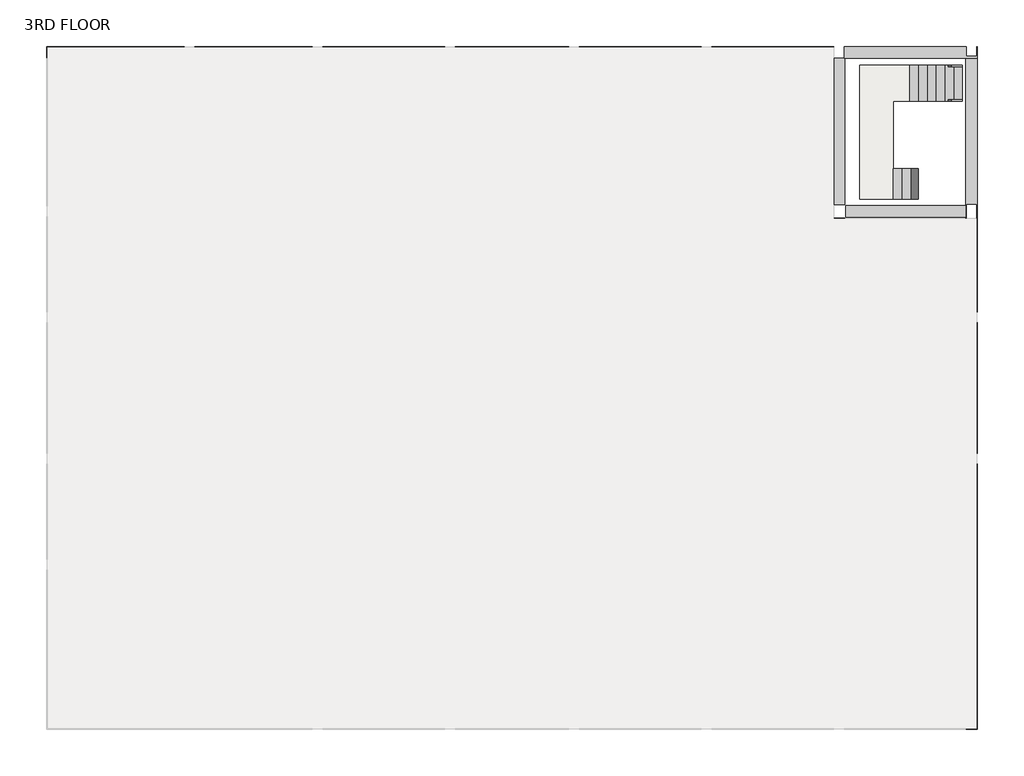
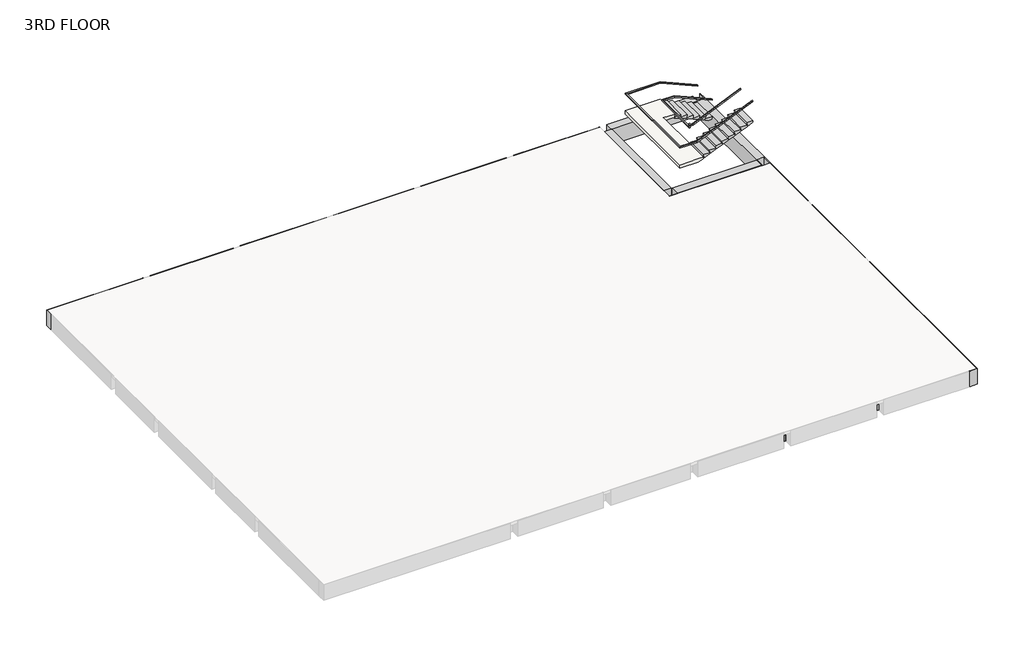
# One storey, part 2 of 2: 5 beams, 2 railings, 2 stair flights, 1 slab.
"""IFC4 building model written with IfcOpenShell, lengths in millimetres."""

from ifc_helpers import new_model, si_unit, frame, origin, place, context, project, spatial, polyline, outline, extrude, faceted_brep, element, save

model = new_model("IFC4")

# Units and contexts
model_context = context("Model", 3, world=origin())
ifc_project = project(units=[si_unit("LENGTHUNIT", "METRE", prefix="MILLI")], contexts=[model_context])

# Site, building, storey
site = spatial("IfcSite", under=ifc_project)
building = spatial("IfcBuilding", under=site)
storey = spatial("IfcBuildingStorey", under=building, Name="3RD FLOOR", Elevation=10668.0)

# Beams
placement = place(None, origin())
element("IfcBeam", 1, ObjectType="M_Concrete-Rectangular Beam : 400 x 800mm", at=placement, inside=storey, context=model_context, shape_type="Brep", body=[
    faceted_brep([(6397.6508981, 16716.9690835, 10668.0), (6397.6508981, 17116.9690835, 10668.0), (6375.4508981, 17116.9690835, 10668.0), (6375.4508981, 16789.9690835, 10668.0), (6019.8508981, 16789.9690835, 10668.0), (6019.8508981, 17116.9690835, 10668.0), (1803.4508981, 17116.9690835, 10668.0), (1803.4508981, 16716.9690835, 10668.0), (1825.6508981, 16716.9690835, 10668.0), (5997.6508981, 16716.9690835, 10668.0), (6397.6508981, 16716.9690835, 9868.0), (1803.4508981, 16716.9690835, 9868.0), (1825.6508981, 16716.9690835, 9868.0), (5997.6508981, 16716.9690835, 9868.0), (6397.6508981, 17116.9690835, 9868.0), (1803.4508981, 17116.9690835, 9868.0), (6019.8508981, 17116.9690835, 9868.0), (6019.8508981, 16789.9690835, 9868.0), (6375.4508981, 16789.9690835, 9868.0), (6375.4508981, 17116.9690835, 9868.0)], [[[0, 1, 2, 3, 4, 5, 6, 7, 8, 9]], [[10, 0, 9, 8, 7, 11, 12, 13]], [[14, 10, 13, 12, 11, 15, 16, 17, 18, 19]], [[1, 14, 19, 2]], [[1, 0, 10, 14]], [[18, 3, 2, 19]], [[3, 18, 17, 4]], [[4, 17, 16, 5]], [[5, 16, 15, 6]], [[7, 6, 15, 11]]]),
    faceted_brep([(-25701.5491019, 16716.9690835, 10668.0), (-25701.5491019, 17116.9690835, 10668.0), (-25701.5491019, 17116.9690835, 9868.0), (-25701.5491019, 16716.9690835, 9868.0), (-25323.7491019, 17094.7690835, 9868.0), (-25323.7491019, 16739.1690835, 9868.0), (-25323.7491019, 16739.1690835, 10515.6), (-25323.7491019, 17094.7690835, 10515.6), (-25679.3491019, 16739.1690835, 9868.0), (-25679.3491019, 16739.1690835, 10515.6), (-25679.3491019, 16716.9690835, 10668.0), (-25679.3491019, 16716.9690835, 10515.6), (-25679.3491019, 17094.7690835, 9868.0), (-25679.3491019, 17094.7690835, 10515.6), (-25679.3491019, 17094.7690835, 10668.0), (-20954.9491019, 16716.9690835, 9868.0), (-20954.9491019, 17116.9690835, 9868.0), (-20954.9491019, 17116.9690835, 10668.0), (-20954.9491019, 17094.7690835, 10668.0), (-20954.9491019, 17094.7690835, 10515.6), (-20954.9491019, 16716.9690835, 10515.6), (-25301.5491019, 16716.9690835, 9868.0), (-20977.1491019, 16716.9690835, 9868.0), (-20977.1491019, 16716.9690835, 10515.6), (-25301.5491019, 16716.9690835, 10515.6)], [[[0, 1, 2, 3]], [[4, 5, 6, 7]], [[5, 8, 9, 6]], [[10, 11, 9, 8, 12, 13, 14]], [[15, 16, 17, 18, 19, 20]], [[1, 0, 10, 14, 18, 17]], [[0, 3, 21, 22, 15, 20, 23, 24, 11, 10]], [[3, 2, 16, 15, 22, 21], [5, 4, 12, 8]], [[2, 1, 17, 16]], [[14, 13, 12, 4, 7, 19, 18]], [[19, 7, 6, 9, 11, 24, 23, 20]]]),
    faceted_brep([(-2768.5491019, 17094.7690835, 10515.6), (1447.8508981, 17094.7690835, 10515.6), (1447.8508981, 17094.7690835, 10668.0), (-2768.5491019, 17094.7690835, 10668.0), (-2768.5491019, 17116.9690835, 9868.0), (-2768.5491019, 16716.9690835, 9868.0), (-2768.5491019, 16716.9690835, 10515.6), (-2768.5491019, 17116.9690835, 10668.0), (1447.8508981, 16716.9690835, 9868.0), (1447.8508981, 17116.9690835, 9868.0), (1447.8508981, 17116.9690835, 10668.0), (1447.8508981, 16716.9690835, 10515.6), (-2746.3491019, 16716.9690835, 9868.0), (1425.6508981, 16716.9690835, 9868.0), (1425.6508981, 16716.9690835, 10515.6), (-2746.3491019, 16716.9690835, 10515.6)], [[[0, 1, 2, 3]], [[4, 5, 6, 0, 3, 7]], [[8, 9, 10, 2, 1, 11]], [[10, 7, 3, 2]], [[5, 12, 13, 8, 11, 14, 15, 6]], [[5, 4, 9, 8, 13, 12]], [[4, 7, 10, 9]], [[1, 0, 6, 15, 14, 11]]]),
    faceted_brep([(-16179.7491019, 17116.9690835, 9868.0), (-16179.7491019, 16716.9690835, 9868.0), (-16179.7491019, 16716.9690835, 10515.6), (-16179.7491019, 17094.7690835, 10515.6), (-16179.7491019, 17094.7690835, 10668.0), (-16179.7491019, 17116.9690835, 10668.0), (-11963.3491019, 16716.9690835, 9868.0), (-11963.3491019, 17116.9690835, 9868.0), (-11963.3491019, 17116.9690835, 10668.0), (-11963.3491019, 17094.7690835, 10668.0), (-11963.3491019, 17094.7690835, 10515.6), (-11963.3491019, 16716.9690835, 10515.6), (-16157.5491019, 16716.9690835, 9868.0), (-11985.5491019, 16716.9690835, 9868.0), (-11985.5491019, 16716.9690835, 10515.6), (-16157.5491019, 16716.9690835, 10515.6)], [[[0, 1, 2, 3, 4, 5]], [[6, 7, 8, 9, 10, 11]], [[8, 5, 4, 9]], [[1, 12, 13, 6, 11, 14, 15, 2]], [[1, 0, 7, 6, 13, 12]], [[0, 5, 8, 7]], [[3, 10, 9, 4]], [[10, 3, 2, 15, 14, 11]]]),
    faceted_brep([(-16535.3491019, 16716.9690835, 9868.0), (-16535.3491019, 17116.9690835, 9868.0), (-16535.3491019, 17116.9690835, 10668.0), (-16535.3491019, 17094.7690835, 10668.0), (-16535.3491019, 17094.7690835, 10515.6), (-16535.3491019, 16716.9690835, 10515.6), (-20599.3491019, 17116.9690835, 10668.0), (-20599.3491019, 17094.7690835, 10668.0), (-20599.3491019, 16716.9690835, 9868.0), (-20577.1491019, 16716.9690835, 9868.0), (-16557.5491019, 16716.9690835, 9868.0), (-16557.5491019, 16716.9690835, 10515.6), (-20577.1491019, 16716.9690835, 10515.6), (-20599.3491019, 16716.9690835, 10515.6), (-20599.3491019, 17116.9690835, 9868.0), (-20599.3491019, 17094.7690835, 10515.6)], [[[0, 1, 2, 3, 4, 5]], [[2, 6, 7, 3]], [[8, 9, 10, 0, 5, 11, 12, 13]], [[1, 0, 10, 9, 8, 14]], [[2, 1, 14, 6]], [[14, 8, 13, 15, 7, 6]], [[15, 4, 3, 7]], [[4, 15, 13, 12, 11, 5]]]),
    faceted_brep([(-11607.7491019, 17116.9690835, 9868.0), (-11607.7491019, 16716.9690835, 9868.0), (-11607.7491019, 16716.9690835, 10515.6), (-11607.7491019, 17094.7690835, 10515.6), (-11607.7491019, 17094.7690835, 10668.0), (-11607.7491019, 17116.9690835, 10668.0), (-7696.1491019, 16716.9690835, 9868.0), (-7696.1491019, 17116.9690835, 9868.0), (-7696.1491019, 17116.9690835, 10668.0), (-7696.1491019, 17094.7690835, 10668.0), (-7696.1491019, 17094.7690835, 10515.6), (-7696.1491019, 16716.9690835, 10515.6), (-11585.5491019, 16716.9690835, 9868.0), (-7718.3491019, 16716.9690835, 9868.0), (-7718.3491019, 16716.9690835, 10515.6), (-11585.5491019, 16716.9690835, 10515.6)], [[[0, 1, 2, 3, 4, 5]], [[6, 7, 8, 9, 10, 11]], [[8, 5, 4, 9]], [[1, 12, 13, 6, 11, 14, 15, 2]], [[1, 0, 7, 6, 13, 12]], [[0, 5, 8, 7]], [[3, 10, 9, 4]], [[10, 3, 2, 15, 14, 11]]]),
    faceted_brep([(-7340.5491019, 17116.9690835, 9868.0), (-7340.5491019, 16716.9690835, 9868.0), (-7340.5491019, 16716.9690835, 10515.6), (-7340.5491019, 17094.7690835, 10515.6), (-7340.5491019, 17094.7690835, 10668.0), (-7340.5491019, 17116.9690835, 10668.0), (-3124.1491019, 16716.9690835, 9868.0), (-3124.1491019, 17116.9690835, 9868.0), (-3124.1491019, 17116.9690835, 10668.0), (-3124.1491019, 17094.7690835, 10668.0), (-3124.1491019, 17094.7690835, 10515.6), (-3124.1491019, 16716.9690835, 10515.6), (-7318.3491019, 16716.9690835, 9868.0), (-3146.3491019, 16716.9690835, 9868.0), (-3146.3491019, 16716.9690835, 10515.6), (-7318.3491019, 16716.9690835, 10515.6)], [[[0, 1, 2, 3, 4, 5]], [[6, 7, 8, 9, 10, 11]], [[8, 5, 4, 9]], [[1, 12, 13, 6, 11, 14, 15, 2]], [[1, 0, 7, 6, 13, 12]], [[0, 5, 8, 7]], [[3, 10, 9, 4]], [[10, 3, 2, 15, 14, 11]]]),
])
element("IfcBeam", 2, ObjectType="M_Concrete-Rectangular Beam : 400 x 800mm", at=placement, inside=storey, context=model_context, shape_type="Brep", body=[
    faceted_brep([(5997.6508981, -6447.8309165, 10668.0), (6397.6508981, -6447.8309165, 10668.0), (6397.6508981, 2718.3690835, 10668.0), (6375.4508981, 2718.3690835, 10668.0), (6375.4508981, -6425.6309165, 10668.0), (5997.6508981, -6425.6309165, 10668.0), (5997.6508981, -6447.8309165, 9868.0), (5997.6508981, -6425.6309165, 10515.6), (5997.6508981, -6047.8309165, 10515.6), (5997.6508981, -961.4309165, 10515.6), (5997.6508981, -561.4309165, 10515.6), (5997.6508981, 2696.1690835, 10515.6), (5997.6508981, 2718.3690835, 10515.6), (5997.6508981, 2718.3690835, 9868.0), (5997.6508981, 2696.1690835, 9868.0), (5997.6508981, -561.4309165, 9868.0), (5997.6508981, -961.4309165, 9868.0), (5997.6508981, -6047.8309165, 9868.0), (6397.6508981, -6447.8309165, 9868.0), (6397.6508981, 2718.3690835, 9868.0), (6375.4508981, -6425.6309165, 9868.0), (6375.4508981, -6070.0309165, 9868.0), (6019.8508981, -6070.0309165, 9868.0), (6019.8508981, -6425.6309165, 9868.0), (6375.4508981, -1015.4309165, 9868.0), (6375.4508981, -507.4309165, 9868.0), (6019.8508981, -507.4309165, 9868.0), (6019.8508981, -1015.4309165, 9868.0), (6375.4508981, 2718.3690835, 10515.6), (6375.4508981, -507.4309165, 10515.6), (6375.4508981, -1015.4309165, 10515.6), (6375.4508981, -6070.0309165, 10515.6), (6375.4508981, -6425.6309165, 10515.6), (6019.8508981, -6425.6309165, 10515.6), (6019.8508981, -6070.0309165, 10515.6), (6019.8508981, -1015.4309165, 10515.6), (6019.8508981, -507.4309165, 10515.6)], [[[0, 1, 2, 3, 4, 5]], [[6, 0, 5, 7, 8, 9, 10, 11, 12, 13, 14, 15, 16, 17]], [[18, 6, 17, 16, 15, 14, 13, 19], [20, 21, 22, 23], [24, 25, 26, 27]], [[1, 18, 19, 2]], [[1, 0, 6, 18]], [[3, 28, 29, 25, 24, 30, 31, 21, 20, 32, 4]], [[4, 32, 20, 23, 33, 7, 5]], [[23, 22, 34, 33]], [[22, 21, 31, 34]], [[19, 13, 12, 28, 3, 2]], [[24, 27, 35, 30]], [[27, 26, 36, 35]], [[26, 25, 29, 36]], [[31, 30, 35, 36, 29, 28, 12, 11, 10, 9, 8, 7, 33, 34]]]),
    faceted_brep([(5997.6508981, 16716.9690835, 9868.0), (5997.6508981, 16716.9690835, 10668.0), (6397.6508981, 16716.9690835, 10668.0), (6397.6508981, 16716.9690835, 9868.0), (5997.6508981, 7950.7690835, 9868.0), (6397.6508981, 7950.7690835, 9868.0), (6397.6508981, 7950.7690835, 10668.0), (6375.4508981, 7950.7690835, 10668.0), (6375.4508981, 7950.7690835, 10515.6), (5997.6508981, 7950.7690835, 10515.6), (5997.6508981, 11630.5690835, 10668.0), (5997.6508981, 11230.5690835, 10668.0), (5997.6508981, 11176.5690835, 10668.0), (6019.8508981, 11176.5690835, 10668.0), (6019.8508981, 11684.5690835, 10668.0), (6375.4508981, 11684.5690835, 10668.0), (6375.4508981, 11176.5690835, 10668.0), (5997.6508981, 11630.5690835, 9868.0), (5997.6508981, 11230.5690835, 9868.0), (5997.6508981, 7972.9690835, 9868.0), (5997.6508981, 7972.9690835, 10515.6), (5997.6508981, 11176.5690835, 10515.6), (6375.4508981, 11176.5690835, 9868.0), (6375.4508981, 11684.5690835, 9868.0), (6019.8508981, 11684.5690835, 9868.0), (6019.8508981, 11176.5690835, 9868.0), (6019.8508981, 11176.5690835, 10515.6), (6375.4508981, 11176.5690835, 10515.6)], [[[0, 1, 2, 3]], [[4, 5, 6, 7, 8, 9]], [[2, 1, 10, 11, 12, 13, 14, 15, 16, 7, 6]], [[1, 0, 17, 18, 19, 4, 9, 20, 21, 12, 11, 10]], [[0, 3, 5, 4, 19, 18, 17], [22, 23, 24, 25]], [[3, 2, 6, 5]], [[22, 25, 26, 27]], [[24, 14, 13, 26, 25]], [[14, 24, 23, 15]], [[8, 27, 26, 21, 20, 9]], [[27, 8, 7, 16, 15, 23, 22]], [[21, 26, 13, 12]]]),
    faceted_brep([(6397.6508981, 7595.1690835, 9868.0), (5997.6508981, 7595.1690835, 9868.0), (5997.6508981, 7595.1690835, 10515.6), (6375.4508981, 7595.1690835, 10515.6), (6375.4508981, 7595.1690835, 10668.0), (6397.6508981, 7595.1690835, 10668.0), (5997.6508981, 3073.9690835, 9868.0), (6397.6508981, 3073.9690835, 9868.0), (6397.6508981, 3073.9690835, 10668.0), (6375.4508981, 3073.9690835, 10668.0), (6375.4508981, 3073.9690835, 10515.6), (5997.6508981, 3073.9690835, 10515.6), (5997.6508981, 7572.9690835, 9868.0), (5997.6508981, 3096.1690835, 9868.0), (5997.6508981, 3096.1690835, 10515.6), (5997.6508981, 7572.9690835, 10515.6)], [[[0, 1, 2, 3, 4, 5]], [[6, 7, 8, 9, 10, 11]], [[8, 5, 4, 9]], [[1, 12, 13, 6, 11, 14, 15, 2]], [[1, 0, 7, 6, 13, 12]], [[0, 5, 8, 7]], [[3, 10, 9, 4]], [[10, 3, 2, 15, 14, 11]]]),
])
element("IfcBeam", 3, ObjectType="M_Concrete-Rectangular Beam : 400 x 800mm", at=placement, inside=storey, context=model_context, shape_type="SweptSolid", body=[
    extrude(outline(polyline([(-2746.3491019, -6047.8309165), (-2768.5491019, -6047.8309165), (-2768.5491019, -6019.2309165), (-3124.1491019, -6019.2309165), (-3124.1491019, -6047.8309165), (-3146.3491019, -6047.8309165), (-3146.3491019, -990.0309165), (-2746.3491019, -990.0309165), (-2746.3491019, -6047.8309165)])), frame((0.0, 0.0, 9868.0), z_axis=(0.0, 0.0, 1.0), x_axis=(1.0, 0.0, 0.0)), (0.0, 0.0, 1.0), 647.6),
    extrude(outline(polyline([(-2768.5491019, 16716.9690835), (-2746.3491019, 16716.9690835), (-2746.3491019, 11659.1690835), (-3146.3491019, 11659.1690835), (-3146.3491019, 16716.9690835), (-3124.1491019, 16716.9690835), (-3124.1491019, 16688.3690835), (-2768.5491019, 16688.3690835), (-2768.5491019, 16716.9690835)])), frame((0.0, 0.0, 9868.0), z_axis=(0.0, 0.0, 1.0), x_axis=(1.0, 0.0, 0.0)), (0.0, 0.0, 1.0), 647.6),
    extrude(outline(polyline([(-3146.3491019, 11201.9690835), (-2746.3491019, 11201.9690835), (-2746.3491019, 8001.5690835), (-3146.3491019, 8001.5690835), (-3146.3491019, 11201.9690835)])), frame((0.0, 0.0, 9868.0), z_axis=(0.0, 0.0, 1.0), x_axis=(1.0, 0.0, 0.0)), (0.0, 0.0, 1.0), 647.6),
    extrude(outline(polyline([(-3146.3491019, 7544.3690835), (-2746.3491019, 7544.3690835), (-2746.3491019, 3124.7690835), (-3146.3491019, 3124.7690835), (-3146.3491019, 7544.3690835)])), frame((0.0, 0.0, 9868.0), z_axis=(0.0, 0.0, 1.0), x_axis=(1.0, 0.0, 0.0)), (0.0, 0.0, 1.0), 647.6),
    extrude(outline(polyline([(-2746.3491019, -532.8309165), (-3146.3491019, -532.8309165), (-3146.3491019, 2667.5690835), (-2746.3491019, 2667.5690835), (-2746.3491019, -532.8309165)])), frame((0.0, 0.0, 9868.0), z_axis=(0.0, 0.0, 1.0), x_axis=(1.0, 0.0, 0.0)), (0.0, 0.0, 1.0), 647.6),
])
element("IfcBeam", 4, ObjectType="M_Concrete-Rectangular Beam : 400 x 800mm", at=placement, inside=storey, context=model_context, shape_type="Brep", body=[
    faceted_brep([(1425.6508981, -990.0309165, 9868.0), (1425.6508981, -6047.8309165, 9868.0), (1425.6508981, -6047.8309165, 10515.6), (1425.6508981, -990.0309165, 10515.6), (1825.6508981, -6047.8309165, 9868.0), (1803.4508981, -6047.8309165, 9868.0), (1803.4508981, -6019.2309165, 9868.0), (1447.8508981, -6019.2309165, 9868.0), (1447.8508981, -6047.8309165, 9868.0), (1825.6508981, -990.0309165, 9868.0), (1825.6508981, -990.0309165, 10515.6), (1825.6508981, -6047.8309165, 10515.6), (1447.8508981, -6047.8309165, 10515.6), (1803.4508981, -6047.8309165, 10515.6), (1803.4508981, -6019.2309165, 10515.6), (1447.8508981, -6019.2309165, 10515.6)], [[[0, 1, 2, 3]], [[4, 5, 6, 7, 8, 1, 0, 9]], [[4, 9, 10, 11]], [[1, 8, 12, 2]], [[6, 5, 13, 14]], [[8, 7, 15, 12]], [[7, 6, 14, 15]], [[5, 4, 11, 13]], [[9, 0, 3, 10]], [[3, 2, 12, 15, 14, 13, 11, 10]]]),
    faceted_brep([(1825.6508981, 16716.9690835, 10668.0), (1825.6508981, 16716.9690835, 9868.0), (1803.4508981, 16716.9690835, 9868.0), (1803.4508981, 16716.9690835, 10668.0), (1803.4508981, 16713.7690835, 9868.0), (1803.4508981, 16713.7690835, 10668.0), (1447.8508981, 16713.7690835, 9868.0), (1447.8508981, 16713.7690835, 10515.6), (1447.8508981, 16713.7690835, 10668.0), (1447.8508981, 16716.9690835, 9868.0), (1447.8508981, 16716.9690835, 10515.6), (1425.6508981, 16716.9690835, 9868.0), (1425.6508981, 16716.9690835, 10515.6), (1425.6508981, 11659.1690835, 9868.0), (1825.6508981, 11659.1690835, 9868.0), (1825.6508981, 11659.1690835, 10668.0), (1447.8508981, 11659.1690835, 10668.0), (1447.8508981, 11659.1690835, 10515.6), (1425.6508981, 11659.1690835, 10515.6)], [[[0, 1, 2, 3]], [[4, 5, 3, 2]], [[5, 4, 6, 7, 8]], [[6, 9, 10, 7]], [[9, 11, 12, 10]], [[13, 14, 15, 16, 17, 18]], [[0, 3, 5, 8, 16, 15]], [[11, 13, 18, 12]], [[2, 1, 14, 13, 11, 9, 6, 4]], [[1, 0, 15, 14]], [[17, 7, 10, 12, 18]], [[7, 17, 16, 8]]]),
    faceted_brep([(1825.6508981, 11201.9690835, 9868.0), (1425.6508981, 11201.9690835, 9868.0), (1425.6508981, 11201.9690835, 10515.6), (1447.8508981, 11201.9690835, 10515.6), (1447.8508981, 11201.9690835, 10668.0), (1825.6508981, 11201.9690835, 10668.0), (1425.6508981, 8001.5690835, 9868.0), (1825.6508981, 8001.5690835, 9868.0), (1825.6508981, 8001.5690835, 10515.6), (1425.6508981, 8001.5690835, 10515.6), (1447.8508981, 11176.5690835, 10668.0), (1825.6508981, 11176.5690835, 10668.0), (1825.6508981, 11176.5690835, 10515.6), (1447.8508981, 11176.5690835, 10515.6)], [[[0, 1, 2, 3, 4, 5]], [[6, 7, 8, 9]], [[5, 4, 10, 11]], [[1, 6, 9, 2]], [[1, 0, 7, 6]], [[0, 5, 11, 12, 8, 7]], [[12, 13, 3, 2, 9, 8]], [[13, 10, 4, 3]], [[10, 13, 12, 11]]]),
    faceted_brep([(1825.6508981, 7544.3690835, 9868.0), (1425.6508981, 7544.3690835, 9868.0), (1425.6508981, 7544.3690835, 10515.6), (1825.6508981, 7544.3690835, 10515.6), (1425.6508981, 3124.7690835, 9868.0), (1825.6508981, 3124.7690835, 9868.0), (1825.6508981, 3124.7690835, 10515.6), (1425.6508981, 3124.7690835, 10515.6)], [[[0, 1, 2, 3]], [[4, 5, 6, 7]], [[1, 4, 7, 2]], [[1, 0, 5, 4]], [[5, 0, 3, 6]], [[3, 2, 7, 6]]]),
    faceted_brep([(1425.6508981, -532.8309165, 9868.0), (1825.6508981, -532.8309165, 9868.0), (1825.6508981, -532.8309165, 10515.6), (1425.6508981, -532.8309165, 10515.6), (1425.6508981, 2667.5690835, 9868.0), (1425.6508981, 2667.5690835, 10515.6), (1825.6508981, 2667.5690835, 9868.0), (1825.6508981, 2667.5690835, 10515.6)], [[[0, 1, 2, 3]], [[4, 0, 3, 5]], [[1, 0, 4, 6]], [[1, 6, 7, 2]], [[6, 4, 5, 7]], [[3, 2, 7, 5]]]),
])
element("IfcBeam", 5, ObjectType="M_Concrete-Rectangular Beam : 400 x 800mm", at=placement, inside=storey, context=model_context, shape_type="SweptSolid", body=[
    extrude(outline(polyline([(-25301.5491019, 11608.3690835), (-25301.5491019, 11630.5690835), (-21005.7491019, 11630.5690835), (-21005.7491019, 11230.5690835), (-25301.5491019, 11230.5690835), (-25301.5491019, 11252.7690835), (-25247.5491019, 11252.7690835), (-25247.5491019, 11608.3690835), (-25301.5491019, 11608.3690835)])), frame((0.0, 0.0, 9868.0), z_axis=(0.0, 0.0, 1.0), x_axis=(1.0, 0.0, 0.0)), (0.0, 0.0, 1.0), 647.6),
    extrude(outline(polyline([(5997.6508981, 11630.5690835), (5997.6508981, 11230.5690835), (1854.2508981, 11230.5690835), (1854.2508981, 11630.5690835), (5997.6508981, 11630.5690835)])), frame((0.0, 0.0, 9868.0), z_axis=(0.0, 0.0, 1.0), x_axis=(1.0, 0.0, 0.0)), (0.0, 0.0, 1.0), 800.0),
    extrude(outline(polyline([(-20548.5491019, 11230.5690835), (-20548.5491019, 11630.5690835), (-16586.1491019, 11630.5690835), (-16586.1491019, 11230.5690835), (-20548.5491019, 11230.5690835)])), frame((0.0, 0.0, 9868.0), z_axis=(0.0, 0.0, 1.0), x_axis=(1.0, 0.0, 0.0)), (0.0, 0.0, 1.0), 647.6),
    extrude(outline(polyline([(-16128.9491019, 11230.5690835), (-16128.9491019, 11630.5690835), (-12014.1491019, 11630.5690835), (-12014.1491019, 11230.5690835), (-16128.9491019, 11230.5690835)])), frame((0.0, 0.0, 9868.0), z_axis=(0.0, 0.0, 1.0), x_axis=(1.0, 0.0, 0.0)), (0.0, 0.0, 1.0), 647.6),
    extrude(outline(polyline([(-11556.9491019, 11230.5690835), (-11556.9491019, 11630.5690835), (-7746.9491019, 11630.5690835), (-7746.9491019, 11230.5690835), (-11556.9491019, 11230.5690835)])), frame((0.0, 0.0, 9868.0), z_axis=(0.0, 0.0, 1.0), x_axis=(1.0, 0.0, 0.0)), (0.0, 0.0, 1.0), 647.6),
    extrude(outline(polyline([(-7289.7491019, 11230.5690835), (-7289.7491019, 11630.5690835), (-3174.9491019, 11630.5690835), (-3174.9491019, 11230.5690835), (-7289.7491019, 11230.5690835)])), frame((0.0, 0.0, 9868.0), z_axis=(0.0, 0.0, 1.0), x_axis=(1.0, 0.0, 0.0)), (0.0, 0.0, 1.0), 647.6),
    extrude(outline(polyline([(-2717.7491019, 11230.5690835), (-2717.7491019, 11630.5690835), (1397.0508981, 11630.5690835), (1397.0508981, 11230.5690835), (-2717.7491019, 11230.5690835)])), frame((0.0, 0.0, 9868.0), z_axis=(0.0, 0.0, 1.0), x_axis=(1.0, 0.0, 0.0)), (0.0, 0.0, 1.0), 647.6),
])

# Railings
element("IfcRailing", 6, ObjectType="Handrail", at=placement, inside=storey, context=model_context, shape_type="Brep", body=[
    faceted_brep([(5878.2258195, 16426.305974, 11712.575), (5878.2258195, 16426.305974, 11657.3359813), (5878.2258195, 16477.105974, 11657.3359813), (5878.2258195, 16477.105974, 11712.575), (4049.4258195, 16426.305974, 12493.625), (4039.0320197, 16426.305974, 12442.825), (4039.0320197, 16477.105974, 12442.825), (4049.4258195, 16477.105974, 12493.625), (2398.4258195, 16426.305974, 12493.625), (2398.4258195, 16426.305974, 12442.825), (2347.6258195, 16477.105974, 12442.825), (2347.6258195, 16477.105974, 12493.625), (2398.4258195, 11896.1816424, 12493.625), (2398.4258195, 11896.1816424, 12442.825), (2347.6258195, 11845.3816424, 12442.825), (2347.6258195, 11845.3816424, 12493.625), (3188.2923097, 11896.1816424, 12493.625), (3198.6861096, 11896.1816424, 12442.825), (3198.6861096, 11845.3816424, 12442.825), (3188.2923097, 11845.3816424, 12493.625), (5931.4923097, 11896.1816424, 13665.2), (5931.4923097, 11845.3816424, 13665.2), (5931.4923097, 11845.3816424, 13609.9609813), (5931.4923097, 11896.1816424, 13609.9609813)], [[[0, 1, 2, 3]], [[1, 0, 4, 5]], [[2, 1, 5, 6]], [[3, 2, 6, 7]], [[0, 3, 7, 4]], [[5, 4, 8, 9]], [[6, 5, 9, 10]], [[7, 6, 10, 11]], [[4, 7, 11, 8]], [[9, 8, 12, 13]], [[10, 9, 13, 14]], [[11, 10, 14, 15]], [[8, 11, 15, 12]], [[13, 12, 16, 17]], [[14, 13, 17, 18]], [[15, 14, 18, 19]], [[12, 15, 19, 16]], [[20, 21, 22, 23]], [[17, 16, 20, 23]], [[18, 17, 23, 22]], [[19, 18, 22, 21]], [[16, 19, 21, 20]]]),
])
element("IfcRailing", 7, ObjectType="Handrail", at=placement, inside=storey, context=model_context, shape_type="Brep", body=[
    faceted_brep([(5878.2258195, 15223.6852874, 11712.575), (5878.2258195, 15223.6852874, 11657.3359813), (5878.2258195, 15274.4852874, 11657.3359813), (5878.2258195, 15274.4852874, 11712.575), (4049.4258195, 15223.6852874, 12493.625), (4039.0320197, 15223.6852874, 12442.825), (4039.0320197, 15274.4852874, 12442.825), (4049.4258195, 15274.4852874, 12493.625), (3493.0923097, 15223.6852874, 12493.625), (3493.0923097, 15223.6852874, 12442.825), (3442.2923097, 15274.4852874, 12442.825), (3442.2923097, 15274.4852874, 12493.625), (3493.0923097, 12985.9409784, 12493.625), (3493.0923097, 12935.1409784, 12442.825), (3442.2923097, 12935.1409784, 12442.825), (3442.2923097, 12985.9409784, 12493.625), (3493.0923097, 12985.9409784, 12656.34375), (3493.0923097, 12935.1409784, 12605.54375), (3442.2923097, 12935.1409784, 12605.54375), (3442.2923097, 12985.9409784, 12656.34375), (3493.0923097, 12909.7409784, 12656.34375), (3493.0923097, 12909.7409784, 12605.54375), (3442.2923097, 12858.9409784, 12605.54375), (3442.2923097, 12858.9409784, 12656.34375), (3569.2923097, 12909.7409784, 12656.34375), (3579.6861096, 12909.7409784, 12605.54375), (3579.6861096, 12858.9409784, 12605.54375), (3569.2923097, 12858.9409784, 12656.34375), (5931.4923097, 12909.7409784, 13665.2), (5931.4923097, 12858.9409784, 13665.2), (5931.4923097, 12858.9409784, 13609.9609813), (5931.4923097, 12909.7409784, 13609.9609813)], [[[0, 1, 2, 3]], [[1, 0, 4, 5]], [[2, 1, 5, 6]], [[3, 2, 6, 7]], [[0, 3, 7, 4]], [[5, 4, 8, 9]], [[6, 5, 9, 10]], [[7, 6, 10, 11]], [[4, 7, 11, 8]], [[9, 8, 12, 13]], [[10, 9, 13, 14]], [[11, 10, 14, 15]], [[8, 11, 15, 12]], [[13, 12, 16, 17]], [[14, 13, 17, 18]], [[15, 14, 18, 19]], [[12, 15, 19, 16]], [[17, 16, 20, 21]], [[18, 17, 21, 22]], [[19, 18, 22, 23]], [[16, 19, 23, 20]], [[21, 20, 24, 25]], [[22, 21, 25, 26]], [[23, 22, 26, 27]], [[20, 23, 27, 24]], [[28, 29, 30, 31]], [[25, 24, 28, 31]], [[26, 25, 31, 30]], [[27, 26, 30, 29]], [[24, 27, 29, 28]]]),
])

# Slab
element("IfcSlab", 8, ObjectType="7\" Thickness", at=placement, inside=storey, context=model_context, shape_type="Brep", body=[
    faceted_brep([(4049.4258195, 16477.105974, 11579.225), (4049.4258195, 15223.6852874, 11579.225), (4030.3758195, 15223.6852874, 11449.05), (4030.3758195, 16477.105974, 11449.05), (2347.6258195, 16477.105974, 11579.225), (2347.6258195, 11845.3816424, 11579.225), (3257.5052912, 11845.3816424, 11579.225), (3493.0923097, 11845.3816424, 11579.225), (3512.1423097, 11845.3816424, 11579.225), (3512.1423097, 12909.7409784, 11579.225), (3493.0923097, 12909.7409784, 11579.225), (3493.0923097, 15223.6852874, 11579.225), (3980.212838, 15223.6852874, 11579.225), (3980.212838, 16477.105974, 11579.225), (4030.3758195, 15223.6852874, 11380.0012267), (4030.3758195, 16477.105974, 11380.0012267), (3980.212838, 16477.105974, 11401.425), (2347.6258195, 16477.105974, 11401.425), (2347.6258195, 11845.3816424, 11401.425), (3257.5052912, 11845.3816424, 11401.425), (3493.0923097, 11845.3816424, 11502.0402892), (3512.1423097, 11845.3816424, 11510.1762267), (3512.1423097, 12909.7409784, 11510.1762267), (3493.0923097, 12909.7409784, 11502.0402892), (3493.0923097, 12909.7409784, 11401.425), (3493.0923097, 15223.6852874, 11401.425), (3980.212838, 15223.6852874, 11401.425), (3257.5052912, 12909.7409784, 11401.425)], [[[0, 1, 2, 3]], [[4, 5, 6, 7, 8, 9, 10, 11, 12, 1, 0, 13]], [[3, 2, 14, 15]], [[0, 3, 15, 16, 17, 4, 13]], [[5, 4, 17, 18]], [[5, 18, 19, 20, 7, 6]], [[8, 7, 20, 21]], [[9, 8, 21, 22]], [[10, 9, 22, 23]], [[11, 10, 23, 24, 25]], [[2, 1, 12, 11, 25, 26, 14]], [[24, 27, 19, 18, 17, 16, 26, 25]], [[27, 24, 23]], [[26, 16, 15, 14]], [[19, 27, 23, 22, 21, 20]]]),
])

# Stair flights
element("IfcStairFlight", 9, ObjectType="3/4\" Nosing", at=placement, inside=storey, context=model_context, shape_type="Brep", body=[
    faceted_brep([(5878.2258195, 16477.105974, 10798.175), (5878.2258195, 15223.6852874, 10798.175), (5859.1758195, 15223.6852874, 10668.0), (5859.1758195, 16477.105974, 10668.0), (5554.3758195, 16477.105974, 10798.175), (5554.3758195, 15223.6852874, 10798.175), (5554.3758195, 15223.6852874, 10729.1262267), (5697.5006429, 15223.6852874, 10668.0), (5697.5006429, 16477.105974, 10668.0), (5554.3758195, 16477.105974, 10729.1262267), (5573.4258195, 15223.6852874, 10928.35), (5573.4258195, 16477.105974, 10928.35), (5249.5758195, 16477.105974, 10928.35), (5249.5758195, 15223.6852874, 10928.35), (5249.5758195, 15223.6852874, 10859.3012267), (5249.5758195, 16477.105974, 10859.3012267), (5268.6258195, 15223.6852874, 11058.525), (5268.6258195, 16477.105974, 11058.525), (4944.7758195, 16477.105974, 11058.525), (4944.7758195, 15223.6852874, 11058.525), (4944.7758195, 15223.6852874, 10989.4762267), (4944.7758195, 16477.105974, 10989.4762267), (4963.8258195, 15223.6852874, 11188.7), (4963.8258195, 16477.105974, 11188.7), (4639.9758195, 16477.105974, 11188.7), (4639.9758195, 15223.6852874, 11188.7), (4639.9758195, 15223.6852874, 11119.6512267), (4639.9758195, 16477.105974, 11119.6512267), (4659.0258195, 15223.6852874, 11318.875), (4659.0258195, 16477.105974, 11318.875), (4335.1758195, 16477.105974, 11318.875), (4335.1758195, 15223.6852874, 11318.875), (4335.1758195, 15223.6852874, 11249.8262267), (4335.1758195, 16477.105974, 11249.8262267), (4030.3758195, 15223.6852874, 11449.05), (4049.4258195, 15223.6852874, 11449.05), (4354.2258195, 15223.6852874, 11449.05), (4354.2258195, 16477.105974, 11449.05), (4049.4258195, 16477.105974, 11449.05), (4030.3758195, 16477.105974, 11449.05), (4030.3758195, 15223.6852874, 11380.0012267), (4049.4258195, 15223.6852874, 11371.8652892), (4049.4258195, 16477.105974, 11371.8652892), (4030.3758195, 16477.105974, 11380.0012267)], [[[0, 1, 2, 3]], [[1, 0, 4, 5]], [[1, 5, 6, 7, 2]], [[4, 0, 3, 8, 9]], [[10, 11, 12, 13]], [[10, 13, 14, 6, 5]], [[12, 11, 4, 9, 15]], [[5, 4, 11, 10]], [[16, 17, 18, 19]], [[16, 19, 20, 14, 13]], [[18, 17, 12, 15, 21]], [[13, 12, 17, 16]], [[22, 23, 24, 25]], [[22, 25, 26, 20, 19]], [[24, 23, 18, 21, 27]], [[19, 18, 23, 22]], [[28, 29, 30, 31]], [[28, 31, 32, 26, 25]], [[30, 29, 24, 27, 33]], [[25, 24, 29, 28]], [[34, 35, 36, 37, 38, 39]], [[35, 34, 40, 41]], [[38, 37, 30, 33, 42]], [[34, 39, 43, 40]], [[31, 30, 37, 36]], [[3, 2, 7, 8]], [[8, 7, 6, 14, 20, 26, 32, 41, 40, 43, 42, 33, 27, 21, 15, 9]], [[36, 35, 41, 32, 31]], [[39, 38, 42, 43]]]),
])
element("IfcStairFlight", 10, ObjectType="3/4\" Nosing", at=placement, inside=storey, context=model_context, shape_type="Brep", body=[
    faceted_brep([(3493.0923097, 11845.3816424, 11709.4), (3493.0923097, 12909.7409784, 11709.4), (3512.1423097, 12909.7409784, 11579.225), (3512.1423097, 11845.3816424, 11579.225), (3816.9423097, 11845.3816424, 11709.4), (3816.9423097, 12909.7409784, 11709.4), (3816.9423097, 12909.7409784, 11640.3512267), (3512.1423097, 12909.7409784, 11510.1762267), (3512.1423097, 11845.3816424, 11510.1762267), (3816.9423097, 11845.3816424, 11640.3512267), (3797.8923097, 12909.7409784, 11839.575), (3797.8923097, 11845.3816424, 11839.575), (4121.7423097, 11845.3816424, 11839.575), (4121.7423097, 12909.7409784, 11839.575), (4121.7423097, 12909.7409784, 11770.5262267), (4121.7423097, 11845.3816424, 11770.5262267), (4102.6923097, 12909.7409784, 11969.75), (4102.6923097, 11845.3816424, 11969.75), (4426.5423097, 11845.3816424, 11969.75), (4426.5423097, 12909.7409784, 11969.75), (4426.5423097, 12909.7409784, 11900.7012267), (4426.5423097, 11845.3816424, 11900.7012267), (4407.4923097, 12909.7409784, 12099.925), (4407.4923097, 11845.3816424, 12099.925), (4731.3423097, 11845.3816424, 12099.925), (4731.3423097, 12909.7409784, 12099.925), (4731.3423097, 12909.7409784, 12030.8762267), (4731.3423097, 11845.3816424, 12030.8762267), (4712.2923097, 12909.7409784, 12230.1), (4712.2923097, 11845.3816424, 12230.1), (5036.1423097, 11845.3816424, 12230.1), (5036.1423097, 12909.7409784, 12230.1), (5036.1423097, 12909.7409784, 12161.0512267), (5036.1423097, 11845.3816424, 12161.0512267), (5017.0923097, 12909.7409784, 12360.275), (5017.0923097, 11845.3816424, 12360.275), (5340.9423097, 11845.3816424, 12360.275), (5340.9423097, 12909.7409784, 12360.275), (5340.9423097, 12909.7409784, 12291.2262267), (5340.9423097, 11845.3816424, 12291.2262267), (5321.8923097, 12909.7409784, 12490.45), (5321.8923097, 11845.3816424, 12490.45), (5645.7423097, 11845.3816424, 12490.45), (5645.7423097, 12909.7409784, 12490.45), (5645.7423097, 12909.7409784, 12421.4012267), (5645.7423097, 11845.3816424, 12421.4012267), (5626.6923097, 12909.7409784, 12620.625), (5626.6923097, 11845.3816424, 12620.625), (5931.4923097, 11845.3816424, 12620.625), (5931.4923097, 12909.7409784, 12620.625), (5931.4923097, 12909.7409784, 12543.4402892), (5931.4923097, 11845.3816424, 12543.4402892)], [[[0, 1, 2, 3]], [[1, 0, 4, 5]], [[1, 5, 6, 7, 2]], [[3, 2, 7, 8]], [[4, 0, 3, 8, 9]], [[10, 11, 12, 13]], [[10, 13, 14, 6, 5]], [[12, 11, 4, 9, 15]], [[11, 10, 5, 4]], [[16, 17, 18, 19]], [[16, 19, 20, 14, 13]], [[18, 17, 12, 15, 21]], [[17, 16, 13, 12]], [[22, 23, 24, 25]], [[22, 25, 26, 20, 19]], [[24, 23, 18, 21, 27]], [[23, 22, 19, 18]], [[28, 29, 30, 31]], [[28, 31, 32, 26, 25]], [[30, 29, 24, 27, 33]], [[29, 28, 25, 24]], [[34, 35, 36, 37]], [[34, 37, 38, 32, 31]], [[36, 35, 30, 33, 39]], [[35, 34, 31, 30]], [[40, 41, 42, 43]], [[40, 43, 44, 38, 37]], [[42, 41, 36, 39, 45]], [[41, 40, 37, 36]], [[46, 47, 48, 49]], [[46, 49, 50, 44, 43]], [[48, 47, 42, 45, 51]], [[49, 48, 51, 50]], [[47, 46, 43, 42]], [[7, 6, 14, 20, 26, 32, 38, 44, 50, 51, 45, 39, 33, 27, 21, 15, 9, 8]]]),
])

save(model, "model.ifc")

# Revit data of these elements
# Type "M_Concrete-Rectangular Beam : 400 x 800mm"
#   Length [instance default] = 5' - 0"
#   b = 1' - 3.74803"
#   h = 2' - 7.49606"
#   Structural Material [instance default] = Concrete, Cast-in-Place gray
#   Assembly Code = ""
# Type "Handrail"
#   Assembly Code = "C2010400"
#   built-in parameter 1008612 = 0.0416667 (stored number, unit not read)
#   built-in parameter 1008611 = 0.0416667 (stored number, unit not read)
#   built-in parameter 1008609 = 0.333333 (stored number, unit not read)
#   built-in parameter 1008604 = 0.166667 (stored number, unit not read)
#   built-in parameter 1008603 = 0.166667 (stored number, unit not read)
#   Railing Height = 3' - 0"
#   built-in parameter 1008630 = 2
#   built-in parameter 1008610 = 2
#   built-in parameter 1008618 = Baluster - Square : 3/4"
# Elements 1, 2 (IfcBeam, "M_Concrete-Rectangular Beam : 400 x 800mm")
#   Structural Material = Concrete, Cast-in-Place gray
#   Phase Created = New Construction
#   Materials on its faces: "Concrete, Cast-in-Place gray"
# Elements 3, 4, 5 (IfcBeam, "M_Concrete-Rectangular Beam : 400 x 800mm")
#   Comments = ""
#   Structural Material = Concrete, Cast-in-Place gray
#   Phase Created = New Construction
#   Materials on its faces: "Concrete, Cast-in-Place gray"
# Elements 6, 7 (IfcRailing, "Handrail")
#   Phase Created = New Construction
# Element 8 (IfcSlab, "7\" Thickness")
#   Phase Created = New Construction
#   Materials on its faces: "Concrete, Cast-in-Place gray"
# Elements 9, 10 (IfcStairFlight, "3/4\" Nosing")
#   Phase Created = New Construction
#   Materials on its faces: "Concrete, Cast-in-Place gray"
# Materials
#   "Concrete, Cast-in-Place gray": class "Concrete", colour RGB 192 192 192, transparency 0, Description = "Cast-in-place concrete", Cost = 0
